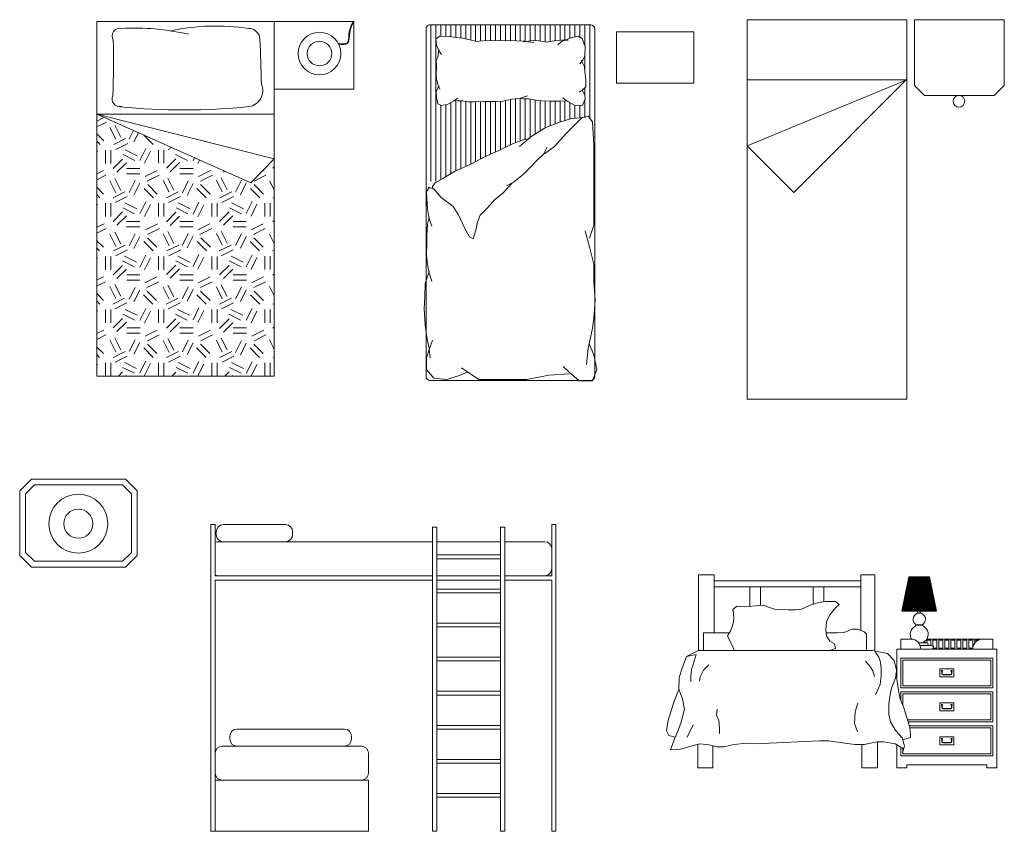
# Model space of a CAD drawing. Units: inches. Extents: x 1994 to 3075, y 3517 to 3950.
# Tile 4 of 58: x 1993.8976 to 1994.1162, y 3553.2299 to 3553.4101. Entities that reach past the tile are written whole.
import ezdxf

# ---------------------------------------------------------------- set-up
doc = ezdxf.new("R2010")
doc.units = ezdxf.units.IN
doc.layers.add('A-FURN-REFR', color=8, linetype='Continuous', lineweight=13)
doc.layers.add('A-FURN-REFR-PATT', color=8, linetype='Continuous', lineweight=13)

# ---------------------------------------------------------------- blocks, each defined once
blk = doc.blocks.new('*X4')
at = {"color": 0, "linetype": 'ByBlock'}
for p, q in [((19.525, 32.20386098788682), (19.525, 32.675)), ((19.55, 32.56810532391988), (19.55, 32.675)), ((19.575, 32.61302412421321), (19.575, 32.675)), ((19.6, 32.61427234615303), (19.6, 32.675)), ((19.625, 32.60794036333506), (19.625, 32.675)), ((19.65, 32.59793129896265), (19.65, 32.675)), ((19.675, 32.59817646525313), (19.675, 32.675)), ((19.7, 32.59593125927973), (19.7, 32.675)), ((19.725, 32.59071820491911), (19.725, 32.675)), ((19.75, 32.58875626807508), (19.75, 32.675)), ((19.775, 32.5935224892048), (19.775, 32.675)), ((19.8, 32.59614861867567), (19.8, 32.675)), ((19.825, 32.59455734515703), (19.825, 32.675)), ((19.85, 32.5927879885456), (19.85, 32.675)), ((19.875, 32.59404453025058), (19.875, 32.675)), ((19.9, 32.59519703632207), (19.9, 32.675)), ((19.925, 32.59638859160449), (19.925, 32.675)), ((19.95, 32.59617959359129), (19.95, 32.675)), ((19.975, 32.59528592712948), (19.975, 32.675)), ((20, 32.59564247452483), (20, 32.675)), ((20.025, 32.59653254351594), (20.025, 32.675)), ((20.05, 32.59544460173633), (20.05, 32.675)), ((20.075, 32.59363490203366), (20.075, 32.675)), ((20.1, 32.59241134187158), (20.1, 32.675)), ((20.125, 32.598098310265), (20.125, 32.675)), ((20.15, 32.60389733444189), (20.15, 32.675)), ((20.175, 32.60912913191685), (20.175, 32.675)), ((20.2, 32.61238895624688), (20.2, 32.675)), ((20.225, 32.61502292055541), (20.225, 32.675)), ((20.25, 32.61658776692677), (20.25, 32.675)), ((20.275, 32.61758867336402), (20.275, 32.675)), ((20.3, 32.60301153474566), (20.3, 32.675)), ((20.325, 32.44626119300636), (20.325, 32.675)), ((20.3, 32.44626119300636), (20.3, 32.59766660268327)), ((19.55, 32.43429497183709), (19.55, 32.5303145499151)), ((20.3, 31.8855920007165), (20.3, 32.44626119300636)), ((20.325, 31.8855920007165), (20.325, 32.44626119300636)), ((19.55, 32.31736883828921), (19.55, 32.3583983061656)), ((19.55, 32.21177313200482), (19.55, 32.29839776882886)), ((19.65, 32.19310101720963), (19.65, 32.29148655342231)), ((19.75, 32.1550408149583), (19.75, 32.29147480162358)), ((19.775, 32.14004617199367), (19.775, 32.2932065184746)), ((19.8, 32.12505152902905), (19.8, 32.29695991761424)), ((19.825, 32.10859105723152), (19.825, 32.30058402418693)), ((19.85, 32.09722511488017), (19.85, 32.30182870692274)), ((19.875, 32.08964787427039), (19.875, 32.30376454748067)), ((19.9, 32.08012334199107), (19.9, 32.30225038066949)), ((19.925, 32.06962839826795), (19.925, 32.2984329992773)), ((19.95, 32.05796084622579), (19.95, 32.29321994491666)), ((20.175, 31.95038486477602), (20.175, 32.2922523717346)), ((20.2, 31.93854186082345), (20.2, 32.29303571994302)), ((19.575, 32.20638032842688), (19.575, 32.26988957351553)), ((19.6, 32.20358354634456), (19.6, 32.27108112879796)), ((19.625, 32.20024132338327), (19.625, 32.28364984065946)), ((19.675, 32.18574866757895), (19.675, 32.29033710469695)), ((19.7, 32.17575223893587), (19.7, 32.29033710469695)), ((19.725, 32.16575581029279), (19.725, 32.29043219075145)), ((19.975, 32.04629329418363), (19.975, 32.28980448432189)), ((20, 32.03487552737632), (20, 32.28861292903947)), ((20.025, 32.02358434798068), (20.025, 32.28842183765934)), ((20.05, 32.01229316858503), (20.05, 32.28842183765934)), ((20.075, 31.99969466619798), (20.075, 32.28784730729937)), ((20.1, 31.98673071948447), (20.1, 32.2869205420797)), ((20.125, 31.97407087268117), (20.125, 32.28650657062169)), ((20.15, 31.9622278687286), (20.15, 32.28908964647222)), ((20.225, 31.92436703603548), (20.225, 32.28364705813529)), ((20.25, 31.90936589769556), (20.25, 32.27313805462554)), ((20.275, 31.89509549871252), (20.275, 32.27050875367903))]:
    blk.add_line(p, q, dxfattribs=at)

msp = doc.modelspace()

# ---------------------------------------------------------------- hatches: boundary and pattern name
at = {"layer": 'A-FURN-REFR-PATT'}
h = msp.add_hatch(dxfattribs=at)
h.set_pattern_fill('GEOL2', color=256, scale=0.0118110236220473, style=0, pattern_type=2)
h.set_pattern_definition([(0, (2000.169371235036, 3548.887718539946), (0.0118110236220473, 0.0118110236220473), [0.0029527559055118, -0.0088582677165354]), (0, (2000.169371235036, 3548.888899642308), (0.0118110236220473, 0.0118110236220473), [0.0029527559055118, -0.0088582677165354]), (90, (2000.176457849209, 3548.890080744671), (-0.0118110236220473, 0.0118110236220473), [0.0029527559055118, -0.0088582677165354]), (90, (2000.177638951571, 3548.890080744671), (-0.0118110236220473, 0.0118110236220473), [0.0029527559055118, -0.0088582677165354]), (45, (2000.178229502752, 3548.888899642308), (0, 0.011811023622272), [0.0029527559055118, -0.0137505538818898]), (45, (2000.179056274406, 3548.888072870655), (0, 0.011811023622272), [0.0029527559055118, -0.0137505538818898]), (135, (2000.175276746847, 3548.894214602938), (-0.011811023622272, 0), [0.0029527559055118, -0.0137505538818898]), (135, (2000.1761035185, 3548.895041374592), (-0.011811023622272, 0), [0.0029527559055118, -0.0137505538818898]), (26.56505119999999, (2000.178229502752, 3548.894214602938), (0.0118110236220484, 4.7252e-12), [0.0029527559055118, -0.0234574957913386]), (26.56505119999999, (2000.178701943697, 3548.893151610812), (0.0118110236220484, 4.7252e-12), [0.0029527559055118, -0.0234574957913386]), (26.56505119999999, (2000.173505093304, 3548.898939012387), (0.0118110236220484, 4.7252e-12), [0.0029527559055118, -0.0234574957913386]), (26.56505119999999, (2000.173977534248, 3548.897876020261), (0.0118110236220484, 4.7252e-12), [0.0029527559055118, -0.0234574957913386]), (63.43494882000001, (2000.172323990941, 3548.890671295851), (6.023e-13, 0.0118110236220484), [0.0029527559055118, -0.0234574957913385]), (63.43494882000001, (2000.173386983067, 3548.890080744671), (6.023e-13, 0.0118110236220484), [0.0029527559055118, -0.0234574957913385]), (63.43494882000001, (2000.171024778343, 3548.894805154119), (6.023e-13, 0.0118110236220484), [0.0029527559055118, -0.0234574957913385]), (63.43494882000001, (2000.169961786217, 3548.8953957053), (6.023e-13, 0.0118110236220484), [0.0029527559055118, -0.0234574957913385]), (116.5650512, (2000.179883046059, 3548.895868146245), (-4.7252e-12, 0.0118110236220484), [0.0029527559055118, -0.0234574957913386]), (116.5650512, (2000.178820053934, 3548.8953957053), (-4.7252e-12, 0.0118110236220484), [0.0029527559055118, -0.0234574957913386]), (153.43494882, (2000.171142888579, 3548.890671295851), (-0.0118110236220484, 6.024e-13), [0.0029527559055118, -0.0234574957913386]), (153.43494882, (2000.171615329524, 3548.891734287977), (-0.0118110236220484, 6.024e-13), [0.0029527559055118, -0.0234574957913386])])
h.paths.add_polyline_path([(1993.954109154694, 3553.379219006938), (1993.948922264658, 3553.373891692003), (1993.914739075954, 3553.389155305615), (1993.914739075954, 3553.330989736288), (1993.954109154694, 3553.330989736288)])
h = msp.add_hatch(dxfattribs=at)
h.set_pattern_fill('ANSI38', color=256, scale=7.66347049375e-05, angle=90, style=0)
h.set_pattern_definition([(135, (0, 0), (-0.0001720498195254, -0.0001720498195254), []), (225, (0, 0), (-0.0001720498195254, -0.0005161494585763), [0.0006082879704418, -0.0003649727822651])])
h.paths.add_polyline_path([(1994.099628953712, 3553.286448017916), (1994.10116164781, 3553.278784547428), (1994.093498177321, 3553.278784547428), (1994.095030871418, 3553.286448017916)])

# ---------------------------------------------------------------- linework, layer by layer
at = {"layer": 'A-FURN-REFR'}
for p, q in [((1993.954109154694, 3553.409729893769), (1993.914739075954, 3553.409729893769)), ((1993.914739075954, 3553.409729893769), (1993.914739075954, 3553.330989736288)), ((1993.954109154694, 3553.394673371351), (1993.954109154694, 3553.409729893769)), ((1993.954109154694, 3553.409729893769), (1993.971825690127, 3553.409729893769)), ((1993.971825690127, 3553.409729893769), (1993.971825690127, 3553.394673371351)), ((1994.059155926548, 3553.325914112681), (1994.059155926548, 3553.410067655988)), ((1994.059155926548, 3553.410067655988), (1994.094588997414, 3553.410067655988)), ((1994.094588997414, 3553.410067655988), (1994.094588997414, 3553.325914112681)), ((1994.0962845141, 3553.410135377998), (1994.116215616461, 3553.410135377998)), ((1994.0962845141, 3553.410135377998), (1994.0962845141, 3553.395519236266)), ((1994.116215616461, 3553.410135377998), (1994.116215616461, 3553.395519236266)), ((1994.059155926548, 3553.396780254413), (1994.094588997414, 3553.396780254413)), ((1994.094588997414, 3553.396780254413), (1994.059155926548, 3553.382103395904)), ((1994.09458426814, 3553.396915934153), (1994.06946382822, 3553.371795494232)), ((1994.094588997414, 3553.396780254413), (1994.094588997414, 3553.396780254413)), ((1994.094588997414, 3553.396780254413), (1994.094588997414, 3553.396780254413)), ((1994.094588997414, 3553.396780254413), (1994.094588997414, 3553.396780254413)), ((1993.971825690127, 3553.394673371351), (1993.954109154694, 3553.394673371351)), ((1993.954109154694, 3553.330989736288), (1993.954109154694, 3553.394673371351)), ((1994.098499081028, 3553.393304669337), (1994.0962845141, 3553.395519236266)), ((1994.114001049533, 3553.393304669337), (1994.116215616461, 3553.395519236266)), ((1994.098499081028, 3553.393304669337), (1994.114001049533, 3553.393304669337)), ((1993.914739075954, 3553.389155305615), (1993.948922264658, 3553.373891692003)), ((1993.914739075954, 3553.389155305615), (1993.954119737166, 3553.379216336113)), ((1993.954109154694, 3553.389155305615), (1993.914739075954, 3553.389155305615)), ((1994.059155926548, 3553.382103395904), (1994.06946382822, 3553.371795494232)), ((1993.948922264658, 3553.373891692003), (1993.954109154694, 3553.379219006938)), ((1993.914739075954, 3553.330989736288), (1993.954109154694, 3553.330989736288)), ((1994.094588997414, 3553.325914112681), (1994.059155926548, 3553.325914112681)), ((1993.900243127395, 3553.308154526741), (1993.897632269542, 3553.305543668888)), ((1993.900895841858, 3553.306849097815), (1993.898937698468, 3553.304890954425)), ((1993.921129990221, 3553.308154526741), (1993.900243127395, 3553.308154526741)), ((1993.920477275758, 3553.306849097815), (1993.900895841858, 3553.306849097815)), ((1993.922435419148, 3553.304890954425), (1993.920477275758, 3553.306849097815)), ((1993.923740848074, 3553.305543668888), (1993.921129990221, 3553.308154526741)), ((1993.897632269542, 3553.305543668888), (1993.897632269542, 3553.291183950694)), ((1993.898937698468, 3553.304890954425), (1993.898937698468, 3553.291836665158)), ((1993.922435419148, 3553.291836665158), (1993.922435419148, 3553.304890954425)), ((1993.923740848074, 3553.291183950694), (1993.923740848074, 3553.305543668888)), ((1993.989260282976, 3553.297440995406), (1993.990205889731, 3553.297440995406)), ((1994.004404726865, 3553.297440995406), (1994.005350333621, 3553.297440995406)), ((1993.897632269542, 3553.291183950694), (1993.900243127395, 3553.288573092841)), ((1993.898937698468, 3553.291836665158), (1993.900895841858, 3553.289878521769)), ((1993.920477275758, 3553.289878521769), (1993.922435419148, 3553.291836665158)), ((1993.921129990221, 3553.288573092841), (1993.923740848074, 3553.291183950694)), ((1993.900895841858, 3553.289878521769), (1993.920477275758, 3553.289878521769)), ((1993.900243127395, 3553.288573092841), (1993.921129990221, 3553.288573092841)), ((1994.051841460532, 3553.286859217838), (1994.048294257176, 3553.286859217838)), ((1994.048294257176, 3553.286859217838), (1994.048294257176, 3553.27005170713)), ((1994.051841460532, 3553.274014635587), (1994.051841460532, 3553.286859217838)), ((1994.084390635564, 3553.274536402606), (1994.084390635564, 3553.286859217838)), ((1994.084390635564, 3553.286859217838), (1994.087457124975, 3553.286859217838)), ((1994.087457124975, 3553.286859217838), (1994.087457124975, 3553.269935694535)), ((1994.051841460532, 3553.285558051226), (1994.084390635564, 3553.285558051226)), ((1994.093498177321, 3553.278784547427), (1994.095030871418, 3553.286448017916)), ((1994.099628953712, 3553.286448017916), (1994.095030871418, 3553.286448017916)), ((1994.099628953712, 3553.286448017916), (1994.10116164781, 3553.278784547427)), ((1994.084390635564, 3553.284195219957), (1994.051841460532, 3553.284195219957)), ((1994.059755020064, 3553.284195219957), (1994.059755020064, 3553.279932083761)), ((1994.062088181079, 3553.284195219957), (1994.062088181079, 3553.280069509611)), ((1994.073807242988, 3553.284195219957), (1994.073807242988, 3553.280381305924)), ((1994.076140404003, 3553.284195219957), (1994.076140404003, 3553.280903425881)), ((1994.058479080529, 3553.279808747126), (1994.062797378561, 3553.280120750106)), ((1994.062797378561, 3553.280120750106), (1994.063629812153, 3553.279808747126)), ((1994.072006255235, 3553.279652745637), (1994.073098841809, 3553.28017275422)), ((1994.073098841809, 3553.28017275422), (1994.075053706907, 3553.280748262081)), ((1994.075053706907, 3553.280748262081), (1994.076510484098, 3553.280956267685)), ((1994.076510484098, 3553.280956267685), (1994.07874766134, 3553.280956267685)), ((1994.07874766134, 3553.280956267685), (1994.079580109657, 3553.280280257612)), ((1994.079580109657, 3553.280280257612), (1994.07874766134, 3553.279552232571)), ((1994.055981765029, 3553.279184730314), (1994.056866232162, 3553.279912744502)), ((1994.056085817387, 3553.278352707899), (1994.055981765029, 3553.279184730314)), ((1994.056137850929, 3553.277000676899), (1994.056085817387, 3553.278352707899)), ((1994.056866232162, 3553.279912744502), (1994.058479080529, 3553.279808747126)), ((1994.063629812153, 3553.279808747126), (1994.065190641703, 3553.279288727689)), ((1994.065190641703, 3553.279288727689), (1994.066751471252, 3553.279184730314)), ((1994.066751471252, 3553.279184730314), (1994.068260267261, 3553.279080722085)), ((1994.068260267261, 3553.279080722085), (1994.069873130351, 3553.279080722085)), ((1994.069873130351, 3553.279080722085), (1994.07122584046, 3553.279288727689)), ((1994.07122584046, 3553.279288727689), (1994.072006255235, 3553.279652745637)), ((1994.077446970049, 3553.277992195968), (1994.076718588815, 3553.276432159364)), ((1994.07874766134, 3553.279552232571), (1994.077446970049, 3553.277992195968)), ((1994.10116164781, 3553.278784547427), (1994.093498177321, 3553.278784547427)), ((1994.055409454971, 3553.274400612276), (1994.055929731487, 3553.275752643275)), ((1994.055929731487, 3553.275752643275), (1994.056137850929, 3553.277000676899)), ((1994.076718588815, 3553.276432159364), (1994.076562502916, 3553.274664117156)), ((1994.098128450965, 3553.275752817065), (1994.096531374166, 3553.275752817065)), ((1994.098128450965, 3553.275671139821), (1994.096531374166, 3553.275671139821)), ((1994.09812626846, 3553.275711978443), (1994.096533556671, 3553.275711978443)), ((1994.049432288437, 3553.27005170713), (1994.049432288437, 3553.274014635587)), ((1994.049432288437, 3553.274014635587), (1994.055170395957, 3553.274014635587)), ((1994.054733092555, 3553.27330858014), (1994.055409454971, 3553.274400612276)), ((1994.076562502916, 3553.274664117156), (1994.076770622356, 3553.273364079418)), ((1994.076666562636, 3553.274014098287), (1994.079147556919, 3553.273976101961)), ((1994.079147556919, 3553.273976101961), (1994.080664421513, 3553.274107941238)), ((1994.080664421513, 3553.274107941238), (1994.082445090566, 3553.274833035553)), ((1994.082445090566, 3553.274833035553), (1994.083698150701, 3553.274833035553)), ((1994.083698150701, 3553.274833035553), (1994.085083120427, 3553.27423976966)), ((1994.085083120427, 3553.27423976966), (1994.085610729344, 3553.27371243426)), ((1994.085610729344, 3553.27371243426), (1994.085610729344, 3553.272262245631)), ((1994.056293922104, 3553.27005170713), (1994.054733092555, 3553.27330858014)), ((1994.076770622356, 3553.273364079418), (1994.07749900359, 3553.272168049908)), ((1994.07749900359, 3553.272168049908), (1994.078487523082, 3553.271544033096)), ((1994.078487523082, 3553.271544033096), (1994.07874766134, 3553.270504005076)), ((1994.085610729344, 3553.272262245631), (1994.085610729344, 3553.27005170713)), ((1994.093238606363, 3553.272626038975), (1994.095456045741, 3553.272626038975)), ((1994.093238606363, 3553.272626038975), (1994.093238606363, 3553.270408599597)), ((1994.097192198074, 3553.271788024285), (1994.099015876073, 3553.271788024285)), ((1994.09856046087, 3553.27208270374), (1994.09856046087, 3553.271788024285)), ((1994.099003948745, 3553.271788024285), (1994.099003948745, 3553.272404295037)), ((1994.099003948745, 3553.272404295037), (1994.099890924496, 3553.272404295037)), ((1994.111421609261, 3553.272626038975), (1994.099039287332, 3553.272626038975)), ((1994.099890924496, 3553.272404295037), (1994.099890924496, 3553.271174946646)), ((1994.100334412372, 3553.271085844229), (1994.100334412372, 3553.272404295037)), ((1994.100334412372, 3553.272404295037), (1994.101221388123, 3553.272404295037)), ((1994.101221388123, 3553.272404295037), (1994.101221388123, 3553.270630343535)), ((1994.101664875999, 3553.270630343535), (1994.101664875999, 3553.272404295037)), ((1994.101664875999, 3553.272404295037), (1994.10255185175, 3553.272404295037)), ((1994.10255185175, 3553.272404295037), (1994.10255185175, 3553.270630343535)), ((1994.102995339625, 3553.270630343535), (1994.102995339625, 3553.272404295037)), ((1994.102995339625, 3553.272404295037), (1994.103882315376, 3553.272404295037)), ((1994.103882315376, 3553.272404295037), (1994.103882315376, 3553.270630343535)), ((1994.105212779003, 3553.272404295037), (1994.104325803252, 3553.272404295037)), ((1994.104325803252, 3553.272404295037), (1994.104325803252, 3553.270630343535)), ((1994.105212779003, 3553.270630343535), (1994.105212779003, 3553.272404295037)), ((1994.10654324263, 3553.272404295037), (1994.105656266879, 3553.272404295037)), ((1994.105656266879, 3553.272404295037), (1994.105656266879, 3553.270630343535)), ((1994.10654324263, 3553.270630343535), (1994.10654324263, 3553.272404295037)), ((1994.107873706257, 3553.272404295037), (1994.106986730505, 3553.272404295037)), ((1994.106986730505, 3553.272404295037), (1994.106986730505, 3553.270630343535)), ((1994.107873706257, 3553.270630343535), (1994.107873706257, 3553.272404295037)), ((1994.109204169883, 3553.272404295037), (1994.108317194132, 3553.272404295037)), ((1994.108317194132, 3553.272404295037), (1994.108317194132, 3553.270630343535)), ((1994.109204169883, 3553.270630343535), (1994.109204169883, 3553.272404295037)), ((1994.110455049845, 3553.272404295037), (1994.109647657759, 3553.272404295037)), ((1994.109647657759, 3553.272404295037), (1994.109647657759, 3553.271739063224)), ((1994.111421609261, 3553.272626038975), (1994.113639048639, 3553.272626038975)), ((1994.113639048639, 3553.272626038975), (1994.113639048639, 3553.270408599597)), ((1994.045634156494, 3553.268737970959), (1994.048294257176, 3553.27005170713)), ((1994.045634156494, 3553.268737970959), (1994.047835731839, 3553.269193232193)), ((1994.047835731839, 3553.269193232193), (1994.047152478733, 3553.266992777564)), ((1994.048294257176, 3553.27005170713), (1994.086917560417, 3553.27005170713)), ((1994.07874766134, 3553.270504005076), (1994.077417699342, 3553.27005170713)), ((1994.086917560417, 3553.27005170713), (1994.087980390402, 3553.269823186441)), ((1994.087448975409, 3553.269937446786), (1994.088359967281, 3553.26860913839)), ((1994.087980390402, 3553.269823186441), (1994.090308641991, 3553.269405505543)), ((1994.090308641991, 3553.269405505543), (1994.091776203363, 3553.267850351574)), ((1994.092351630612, 3553.270408599597), (1994.092351630612, 3553.263805254229)), ((1994.092351630612, 3553.270408599597), (1994.11452602439, 3553.270408599597)), ((1994.097536850776, 3553.271174946646), (1994.100088761942, 3553.271174946646)), ((1994.097673485119, 3553.270408599597), (1994.097673485119, 3553.270408599597)), ((1994.101221388123, 3553.270630343535), (1994.100436270846, 3553.270630343535)), ((1994.10255185175, 3553.270630343535), (1994.101664875999, 3553.270630343535)), ((1994.103882315376, 3553.270630343535), (1994.102995339625, 3553.270630343535)), ((1994.104325803252, 3553.270630343535), (1994.105212779003, 3553.270630343535)), ((1994.105656266879, 3553.270630343535), (1994.10654324263, 3553.270630343535)), ((1994.106986730505, 3553.270630343535), (1994.107873706257, 3553.270630343535)), ((1994.108317194132, 3553.270630343535), (1994.109204169883, 3553.270630343535)), ((1994.109204169883, 3553.270408599597), (1994.109204169883, 3553.270408599597)), ((1994.11452602439, 3553.270408599597), (1994.11452602439, 3553.244026942197)), ((1994.044647256609, 3553.265930486877), (1994.045634156494, 3553.268737970959)), ((1994.047152478733, 3553.266992777564), (1994.046772901855, 3553.265854602768)), ((1994.050594363494, 3553.26688483999), (1994.049399844773, 3553.265690927116)), ((1994.086386152786, 3553.266636314378), (1994.085399238177, 3553.267698605065)), ((1994.088359967281, 3553.26860913839), (1994.08873954416, 3553.267470963593)), ((1994.08873954416, 3553.267470963593), (1994.088891389635, 3553.266029284924)), ((1994.091776203363, 3553.267850351574), (1994.092307610993, 3553.265725781053)), ((1994.093238606363, 3553.268412904157), (1994.113639048639, 3553.268412904157)), ((1994.093238606363, 3553.261760586023), (1994.093238606363, 3553.268412904157)), ((1994.093682094239, 3553.262204073899), (1994.093682094239, 3553.267969416282)), ((1994.093682094239, 3553.267969416282), (1994.113195560763, 3553.267969416282)), ((1994.113195560763, 3553.267969416282), (1994.113195560763, 3553.262204073899)), ((1994.113639048639, 3553.268412904157), (1994.113639048639, 3553.261760586023)), ((1994.044039918878, 3553.264109420227), (1994.044647256609, 3553.265930486877)), ((1994.046772901855, 3553.265854602768), (1994.046621071103, 3553.264261166736)), ((1994.049399844773, 3553.265690927116), (1994.048708272779, 3553.264245666448)), ((1994.086993475793, 3553.26557402369), (1994.086386152786, 3553.266636314378)), ((1994.087373052671, 3553.26428409153), (1994.086993475793, 3553.26557402369)), ((1994.088891389635, 3553.266029284924), (1994.088891389635, 3553.264359975639)), ((1994.092307610993, 3553.265725781053), (1994.092079864866, 3553.26390470355)), ((1994.09219373793, 3553.264815242302), (1994.092763117972, 3553.261173103576)), ((1994.101886619936, 3553.265973720841), (1994.104991035065, 3553.265973720841)), ((1994.101886619936, 3553.264199769339), (1994.101886619936, 3553.265973720841)), ((1994.102330107812, 3553.264953698727), (1994.102330107812, 3553.265530232965)), ((1994.102330107812, 3553.265530232965), (1994.102418805387, 3553.265530232965)), ((1994.102418805387, 3553.264953698727), (1994.102418805387, 3553.265530232965)), ((1994.104237105677, 3553.26473195479), (1994.102640549325, 3553.26473195479)), ((1994.104458849615, 3553.265530232965), (1994.10454754719, 3553.265530232965)), ((1994.104458849615, 3553.265530232965), (1994.104458849615, 3553.264953698727)), ((1994.10454754719, 3553.265530232965), (1994.10454754719, 3553.264953698727)), ((1994.104991035065, 3553.265973720841), (1994.104991035065, 3553.264199769339)), ((1994.043964003503, 3553.261529566762), (1994.044039918878, 3553.264109420227)), ((1994.046621071103, 3553.264261166736), (1994.046621071103, 3553.263198876049)), ((1994.048708272779, 3553.264245666448), (1994.04858254714, 3553.263303101368)), ((1994.088663628784, 3553.26253890899), (1994.087600813523, 3553.260262570251)), ((1994.088891389635, 3553.264359975639), (1994.088663628784, 3553.26253890899)), ((1994.092079864866, 3553.26390470355), (1994.091168865633, 3553.26170424892)), ((1994.104991035065, 3553.264199769339), (1994.101886619936, 3553.264199769339)), ((1994.104237105677, 3553.264643257215), (1994.102640549325, 3553.264643257215)), ((1994.043964003503, 3553.261529566762), (1994.042861434263, 3553.258590286822)), ((1994.04479908736, 3553.259329112132), (1994.043964003503, 3553.261529566762)), ((1994.091168865633, 3553.26170424892), (1994.090789288754, 3553.259883182271)), ((1994.092763117972, 3553.261173103576), (1994.093066779475, 3553.259352036927)), ((1994.093238606363, 3553.261760586023), (1994.113639048639, 3553.261760586023)), ((1994.093238606363, 3553.258946101423), (1994.093238606363, 3553.260873610272)), ((1994.093238606363, 3553.260873610272), (1994.113639048639, 3553.260873610272)), ((1994.093682094239, 3553.262204073899), (1994.113195560763, 3553.262204073899)), ((1994.093682094239, 3553.260430122396), (1994.113195560763, 3553.260430122396)), ((1994.093682094239, 3553.257898375558), (1994.093682094239, 3553.260430122396)), ((1994.113195560763, 3553.260430122396), (1994.113195560763, 3553.254664780014)), ((1994.113639048639, 3553.260873610272), (1994.113639048639, 3553.254221292139)), ((1994.042861434263, 3553.258590286822), (1994.041604060084, 3553.254505852612)), ((1994.045254579615, 3553.257052773394), (1994.04479908736, 3553.259329112132)), ((1994.083729070462, 3553.258365619494), (1994.083121747456, 3553.256468668736)), ((1994.090789288754, 3553.259883182271), (1994.090561542627, 3553.258137988876)), ((1994.090561542627, 3553.258137988876), (1994.090561542627, 3553.255861650138)), ((1994.093066779475, 3553.259352036927), (1994.093901848609, 3553.257379212915)), ((1994.101886619936, 3553.256660475454), (1994.101886619936, 3553.258434426957)), ((1994.101886619936, 3553.258434426957), (1994.104991035065, 3553.258434426957)), ((1994.104991035065, 3553.258434426957), (1994.104991035065, 3553.256660475454)), ((1994.044419495758, 3553.253941774585), (1994.045254579615, 3553.257052773394)), ((1994.052354699122, 3553.255699765486), (1994.052480439485, 3553.257082189205)), ((1994.083121747456, 3553.256468668736), (1994.082969916705, 3553.253888826125)), ((1994.093901848609, 3553.257379212915), (1994.095192424721, 3553.253281807527)), ((1994.104991035065, 3553.256660475454), (1994.101886619936, 3553.256660475454)), ((1994.102330107812, 3553.25799093908), (1994.102418805387, 3553.25799093908)), ((1994.102330107812, 3553.257414404843), (1994.102330107812, 3553.25799093908)), ((1994.102418805387, 3553.257414404843), (1994.102418805387, 3553.25799093908)), ((1994.104237105677, 3553.257192660905), (1994.102640549325, 3553.257192660905)), ((1994.104237105677, 3553.25710396333), (1994.102640549325, 3553.25710396333)), ((1994.104458849615, 3553.25799093908), (1994.104458849615, 3553.257414404843)), ((1994.104458849615, 3553.25799093908), (1994.10454754719, 3553.25799093908)), ((1994.10454754719, 3553.25799093908), (1994.10454754719, 3553.257414404843)), ((1994.041604060084, 3553.254505852612), (1994.041226838997, 3553.252243700761)), ((1994.043508511248, 3553.251665446701), (1994.044419495758, 3553.253941774585)), ((1994.052857645849, 3553.254505852612), (1994.052354699122, 3553.255699765486)), ((1994.052983386211, 3553.252809244151), (1994.052857645849, 3553.254505852612)), ((1994.082969916705, 3553.253888826125), (1994.083653155087, 3553.251991875367)), ((1994.090561542627, 3553.255861650138), (1994.090941119505, 3553.254268214106)), ((1994.090941119505, 3553.254268214106), (1994.092155780242, 3553.25221951684)), ((1994.094756824363, 3553.254664780014), (1994.113195560763, 3553.254664780014)), ((1994.094896511507, 3553.254221292139), (1994.113639048639, 3553.254221292139)), ((1994.041226838997, 3553.252243700761), (1994.041729800447, 3553.251238309587)), ((1994.042825258142, 3553.249996126561), (1994.043508511248, 3553.251665446701)), ((1994.047136547695, 3553.253563287532), (1994.045816288611, 3553.250861277041)), ((1994.052983386211, 3553.251678168225), (1994.052983386211, 3553.252809244151)), ((1994.092155780242, 3553.25221951684), (1994.092155780242, 3553.25221951684)), ((1994.092155780242, 3553.25221951684), (1994.09352227173, 3553.250701954063)), ((1994.095175885796, 3553.253334316388), (1994.113639048639, 3553.253334316388)), ((1994.095192424721, 3553.253281807527), (1994.095420185572, 3553.251688371496)), ((1994.09524831006, 3553.252890828512), (1994.113195560763, 3553.252890828512)), ((1994.095420185572, 3553.251688371496), (1994.095420185572, 3553.250777827317)), ((1994.113195560763, 3553.252890828512), (1994.113195560763, 3553.247125486129)), ((1994.113639048639, 3553.253334316388), (1994.113639048639, 3553.246681998254)), ((1994.041729800447, 3553.251238309587), (1994.041729800447, 3553.251238309587)), ((1994.041729800447, 3553.251238309587), (1994.043166884695, 3553.250830786631)), ((1994.042142019759, 3553.248023302549), (1994.042825258142, 3553.249996126561)), ((1994.045816288611, 3553.250861277041), (1994.045816288611, 3553.250861277041)), ((1994.048594900321, 3553.249389107963), (1994.047759816464, 3553.249161466491)), ((1994.050644630192, 3553.249161466491), (1994.048594900321, 3553.249389107963)), ((1994.059071339971, 3553.249540865326), (1994.056186526243, 3553.2492373506)), ((1994.0608265812, 3553.249389107963), (1994.059071339971, 3553.249540865326)), ((1994.059071339971, 3553.249540865326), (1994.059071339971, 3553.249540865326)), ((1994.075153945829, 3553.250019051355), (1994.0608265812, 3553.249389107963)), ((1994.077276189901, 3553.250019051355), (1994.075153945829, 3553.250019051355)), ((1994.080312849104, 3553.24956379012), (1994.077276189901, 3553.250019051355)), ((1994.08304583208, 3553.249184391285), (1994.080312849104, 3553.24956379012)), ((1994.086841645041, 3553.24956379012), (1994.08517149205, 3553.249184391285)), ((1994.088056305778, 3553.249791420738), (1994.086841645041, 3553.24956379012)), ((1994.089422797266, 3553.249791420738), (1994.088056305778, 3553.249791420738)), ((1994.088056305778, 3553.249791420738), (1994.088056305778, 3553.244026942197)), ((1994.09200394949, 3553.249336148648), (1994.089422797266, 3553.249791420738)), ((1994.09352227173, 3553.250701954063), (1994.094053694084, 3553.248805003305)), ((1994.095420185572, 3553.250777827317), (1994.093640674913, 3553.250279305286)), ((1994.101886619936, 3553.250895133072), (1994.104991035065, 3553.250895133072)), ((1994.101886619936, 3553.24912118157), (1994.101886619936, 3553.250895133072)), ((1994.102330107812, 3553.249875110958), (1994.102330107812, 3553.250451645197)), ((1994.102330107812, 3553.250451645197), (1994.102418805387, 3553.250451645197)), ((1994.102418805387, 3553.249875110958), (1994.102418805387, 3553.250451645197)), ((1994.104237105677, 3553.249653367021), (1994.102640549325, 3553.249653367021)), ((1994.104237105677, 3553.249564669445), (1994.102640549325, 3553.249564669445)), ((1994.104458849615, 3553.250451645197), (1994.10454754719, 3553.250451645197)), ((1994.104458849615, 3553.250451645197), (1994.104458849615, 3553.249875110958)), ((1994.10454754719, 3553.250451645197), (1994.10454754719, 3553.249875110958)), ((1994.104991035065, 3553.250895133072), (1994.104991035065, 3553.24912118157)), ((1994.044343580382, 3553.248175059912), (1994.042142019759, 3553.248023302549)), ((1994.047759816464, 3553.249161466491), (1994.044343580382, 3553.248175059912)), ((1994.048142396977, 3553.244026942197), (1994.048142396977, 3553.249265756845)), ((1994.052390713282, 3553.248706205256), (1994.050644630192, 3553.249161466491)), ((1994.051517671737, 3553.248933835873), (1994.051517671737, 3553.244026942197)), ((1994.053984950897, 3553.248706205256), (1994.052390713282, 3553.248706205256)), ((1994.056186526243, 3553.2492373506), (1994.053984950897, 3553.248706205256)), ((1994.08517149205, 3553.249184391285), (1994.08304583208, 3553.249184391285)), ((1994.084594558752, 3553.244026942197), (1994.084594558752, 3553.249184391285)), ((1994.093863898283, 3553.248235921333), (1994.09200394949, 3553.249336148648)), ((1994.092351630612, 3553.249130482628), (1994.092351630612, 3553.244026942197)), ((1994.093238606363, 3553.246681998254), (1994.093238606363, 3553.248605804232)), ((1994.094053694084, 3553.248805003305), (1994.093674102481, 3553.247666839363)), ((1994.093674102481, 3553.247666839363), (1994.093863898283, 3553.248235921333)), ((1994.093674102481, 3553.247666839363), (1994.093674102481, 3553.247666839363)), ((1994.093682094239, 3553.247125486129), (1994.093682094239, 3553.248343465034)), ((1994.104991035065, 3553.24912118157), (1994.101886619936, 3553.24912118157)), ((1994.093238606363, 3553.246681998254), (1994.113639048639, 3553.246681998254)), ((1994.093682094239, 3553.247125486129), (1994.113195560763, 3553.247125486129)), ((1994.051517671737, 3553.244026942197), (1994.048142396977, 3553.244026942197)), ((1994.088056305778, 3553.244026942197), (1994.084594558752, 3553.244026942197)), ((1994.094569069989, 3553.244026942197), (1994.092351630612, 3553.244026942197)), ((1994.094569069989, 3553.244686302814), (1994.094569069989, 3553.244026942197)), ((1994.094569069989, 3553.244686302814), (1994.112308585012, 3553.244686302814)), ((1994.112308585012, 3553.244686302814), (1994.112308585012, 3553.244026942197)), ((1994.112308585012, 3553.244026942197), (1994.11452602439, 3553.244026942197)), ((1993.990205889731, 3553.229935414131), (1993.989260282976, 3553.229935414131)), ((1994.005350333621, 3553.229935414131), (1994.004404726865, 3553.229935414131))]:
    msp.add_line(p, q, dxfattribs=at)
at = {"layer": 'A-FURN-REFR', "extrusion": (2.7404770908e-06, 0, 0.9999999999962449)}
for p, q in [((1994.017663083944, 3553.38745919332, -8.1741843e-08), (1994.014434587808, 3553.38616825607, -7.28942233e-08)), ((1994.019923031239, 3553.388104661945, -8.79351768e-08), (1994.017663083944, 3553.38745919332, -8.1741843e-08)), ((1994.023328786101, 3553.388485668112, -9.726857e-08), (1994.019923031239, 3553.388104661945, -8.79351768e-08)), ((1994.014434587808, 3553.38616825607, -7.28942233e-08), (1994.011206091673, 3553.384231850195, -6.40466036e-08)), ((1994.011206091673, 3553.384231850195, -6.40466036e-08), (1994.008623294764, 3553.381972710007, -5.69685079e-08))]:
    msp.add_line(p, q, dxfattribs=at)
at = {"layer": 'A-FURN-REFR', "extrusion": (0, 1, 2e-16)}
for p, q in [((1993.940088731704, 3553.298019100508), (1993.940088731704, 3553.229935414131)), ((1993.941034338459, 3553.298019100508), (1993.940088731704, 3553.298019100508)), ((1993.941034338459, 3553.298019100508), (1993.941034338459, 3553.286671819445)), ((1993.956634404617, 3553.298019100508), (1993.942837110295, 3553.298019100508)), ((1994.016682878878, 3553.298019100508), (1994.015737272123, 3553.298019100508)), ((1994.015737272123, 3553.298019100508), (1994.015737272123, 3553.286671819445)), ((1994.016682878878, 3553.229935414131), (1994.016682878878, 3553.298019100508)), ((1993.941252782606, 3553.29643477282), (1993.941252782606, 3553.295821001176)), ((1993.958218732305, 3553.295821001176), (1993.958218732305, 3553.29643477282)), ((1993.989260282976, 3553.297440995406), (1993.989260282976, 3553.285726212691)), ((1993.990205889731, 3553.229935414131), (1993.990205889731, 3553.297440995406)), ((1994.005350333621, 3553.297440995406), (1994.004404726865, 3553.297440995406)), ((1994.004404726865, 3553.297440995406), (1994.004404726865, 3553.285148107588)), ((1994.005350333621, 3553.229935414131), (1994.005350333621, 3553.297440995406)), ((1993.989260282976, 3553.294236673487), (1993.941673059392, 3553.294236673487)), ((1994.004404726865, 3553.294236673487), (1993.990205889731, 3553.294236673487)), ((1994.014152944435, 3553.294236673487), (1994.005350333621, 3553.294236673487)), ((1993.989260282976, 3553.286671819445), (1993.941034338459, 3553.286671819445)), ((1994.004404726865, 3553.286671819445), (1993.990205889731, 3553.286671819445)), ((1994.015737272123, 3553.286671819445), (1994.005350333621, 3553.286671819445)), ((1993.941034338459, 3553.247263221547), (1993.941034338459, 3553.285726212691)), ((1993.989260282976, 3553.285726212691), (1993.941034338459, 3553.285726212691)), ((1993.989260282976, 3553.229935414131), (1993.989260282976, 3553.285726212691)), ((1994.004404726865, 3553.285726212691), (1993.990205889731, 3553.285726212691)), ((1994.004404726865, 3553.229935414131), (1994.004404726865, 3553.285148107588)), ((1994.015737272123, 3553.285726212691), (1994.005350333621, 3553.285726212691)), ((1994.015737272123, 3553.229935414131), (1994.015737272123, 3553.285726212691)), ((1993.969714715081, 3553.252629976257), (1993.945856170473, 3553.252629976257)), ((1993.944271842785, 3553.251045648568), (1993.944271842785, 3553.250431876924)), ((1993.97129904277, 3553.250431876924), (1993.97129904277, 3553.251045648568)), ((1993.941034338459, 3553.247263221547), (1993.941034338459, 3553.242867022882)), ((1993.973491853959, 3553.248847549236), (1993.942618666147, 3553.248847549236)), ((1993.975076181648, 3553.242867022882), (1993.975076181648, 3553.247263221547)), ((1993.941034338459, 3553.241282695193), (1993.941034338459, 3553.242867022882)), ((1993.941034338459, 3553.229935414131), (1993.941034338459, 3553.241282695193)), ((1993.975076181648, 3553.241282695193), (1993.941034338459, 3553.241282695193)), ((1993.975076181648, 3553.229935414131), (1993.975076181648, 3553.241282695193)), ((1993.940088731704, 3553.229935414131), (1993.941034338459, 3553.229935414131)), ((1993.941034338459, 3553.229935414131), (1993.975076181648, 3553.229935414131)), ((1994.016682878878, 3553.229935414131), (1994.015737272123, 3553.229935414131))]:
    msp.add_line(p, q, dxfattribs=at)
at = {"layer": 'A-FURN-REFR', "extrusion": (2.7404770908e-06, 0, 0.9999999999962449), "elevation": 0.0054644779825559}
msp.add_lwpolyline([(1993.988716837792, 3553.330030000304, -0.4142135623730951), (1993.987835480637, 3553.330911357459), (1993.987835480637, 3553.408105389229, -0.4142135623730951), (1993.988716837792, 3553.408986746385), (1994.024411802563, 3553.408986746385, -0.4142135623730948), (1994.025293159718, 3553.408105389229), (1994.025293159718, 3553.330911357459, -0.4142135623730948), (1994.024411802563, 3553.330030000304)], format="xyb", close=True, dxfattribs=at)
at = {"layer": 'A-FURN-REFR'}
for points in [[(1994.030126135478, 3553.407469052605), (1994.047254692625, 3553.407469052605), (1994.047254692625, 3553.396026679955), (1994.030126135478, 3553.396026679955)], [(1993.990205889731, 3553.290454246467), (1994.004404726865, 3553.290454246467), (1994.004404726865, 3553.291285674671), (1993.990205889731, 3553.291285674671)], [(1993.990205889731, 3553.282889392425), (1994.004404726865, 3553.282889392425), (1994.004404726865, 3553.28372082063), (1993.990205889731, 3553.28372082063)], [(1993.990205889731, 3553.275324538383), (1994.004404726865, 3553.275324538383), (1994.004404726865, 3553.276155966587), (1993.990205889731, 3553.276155966587)], [(1993.990205889731, 3553.267759684341), (1994.004404726865, 3553.267759684341), (1994.004404726865, 3553.268591112546), (1993.990205889731, 3553.268591112546)], [(1993.990205889731, 3553.260194830299), (1994.004404726865, 3553.260194830299), (1994.004404726865, 3553.261026258504), (1993.990205889731, 3553.261026258504)], [(1993.990205889731, 3553.252629976257), (1994.004404726865, 3553.252629976257), (1994.004404726865, 3553.253461404461), (1993.990205889731, 3553.253461404461)], [(1993.990205889731, 3553.245065122215), (1994.004404726865, 3553.245065122215), (1994.004404726865, 3553.24589655042), (1993.990205889731, 3553.24589655042)], [(1993.990205889731, 3553.237500268173), (1994.004404726865, 3553.237500268173), (1994.004404726865, 3553.238331696378), (1993.990205889731, 3553.238331696378)]]:
    msp.add_lwpolyline(points, close=True, dxfattribs=at)
at = {"layer": 'A-FURN-REFR', "extrusion": (2.7404770908e-06, 0, 0.9999999999962449), "elevation": 0.0054644779825559}
for points in [[(1993.999119262104, 3553.405286545947), (1993.997264105949, 3553.405708554523), (1993.995830576193, 3553.406046161384), (1993.994565696996, 3553.406214964815), (1993.99296351668, 3553.406383768246), (1993.990855384686, 3553.406468169961), (1993.990012131888, 3553.405792956238), (1993.990180782448, 3553.404442528793), (1993.990686734126, 3553.403260904778), (1993.991277011085, 3553.402416887625)], [(1994.011768054071, 3553.4050333408), (1994.009828572636, 3553.405370947661), (1994.007973416481, 3553.405455349377), (1994.006202585606, 3553.405539751092), (1994.003841477772, 3553.405455349377), (1994.002407948016, 3553.405539751092), (1994.000468466581, 3553.405455349377), (1993.998866286265, 3553.405286545947)], [(1994.0193950511, 3553.405568580201), (1994.017923799495, 3553.405624152808), (1994.016658920298, 3553.405539751092), (1994.014635113584, 3553.405117742516), (1994.012864282709, 3553.405455349377), (1994.011683728791, 3553.405539751092), (1994.009369373409, 3553.405221674875)], [(1994.021971412924, 3553.400306844741), (1994.022646015162, 3553.401150861894), (1994.023067641562, 3553.402079280763), (1994.023151966841, 3553.404104921931), (1994.022477364603, 3553.405961759669), (1994.021634111805, 3553.406468169961), (1994.020031931489, 3553.406130563099), (1994.017923799495, 3553.405286545947), (1994.017080546697, 3553.404526930509)], [(1993.990686734126, 3553.403525661056), (1993.990433758287, 3553.401826075616), (1993.990096457168, 3553.401066460179), (1993.990180782448, 3553.399800434448), (1993.990096457168, 3553.39794359671), (1993.990180782448, 3553.397015177842), (1993.990433758287, 3553.395749152111), (1993.990939709966, 3553.394736331527)], [(1994.022248535104, 3553.40113582132), (1994.022983316282, 3553.399631631017), (1994.023067641562, 3553.398534408718), (1994.023320617401, 3553.396761972696), (1994.023320617401, 3553.39524274182), (1994.022477364603, 3553.394483126381), (1994.021802762365, 3553.394061117804)], [(1993.990686734126, 3553.395431040625), (1993.990096457168, 3553.39414551952), (1993.990180782448, 3553.392879493789), (1993.990433758287, 3553.391444664629), (1993.991277011085, 3553.391107057767), (1993.992710540841, 3553.391360262913), (1993.993975420038, 3553.392119878351), (1993.994902998115, 3553.392710690359)], [(1994.022477364603, 3553.394483126381), (1994.023067641562, 3553.393470305797), (1994.023151966841, 3553.392541886927), (1994.022561689882, 3553.391107057767), (1994.020790859007, 3553.391191459482), (1994.018935702852, 3553.392204280066), (1994.018176775334, 3553.392795092074)], [(1994.010334524315, 3553.393217100651), (1994.008816669279, 3553.392710690359), (1994.006877187844, 3553.392457485212), (1994.004853381129, 3553.392035476636), (1994.003082550254, 3553.39195107492), (1994.00063711714, 3553.39195107492), (1993.998360334586, 3553.391866673205), (1993.997179780669, 3553.391866673205), (1993.995999226752, 3553.392119878351), (1993.994818672836, 3553.392119878351), (1993.993906663943, 3553.392204280066)], [(1994.019357329251, 3553.392119878351), (1994.017670823655, 3553.392035476636), (1994.015478366381, 3553.392035476636), (1994.013454559667, 3553.392119878351), (1994.011768054071, 3553.392373083497), (1994.010587500154, 3553.392541886927), (1994.009406946237, 3553.392541886927), (1994.008142067041, 3553.392710690359)], [(1994.024120068728, 3553.361640448325), (1994.025088617569, 3553.364545057137), (1994.025088617569, 3553.37035427476), (1994.025088617569, 3553.376808961009), (1994.025088617569, 3553.382295444322), (1994.024765767955, 3553.38745919332), (1994.023797219114, 3553.388750130571), (1994.02250582066, 3553.388427396258), (1994.020891572592, 3553.386813724696), (1994.018954474911, 3553.384877318821), (1994.016371678003, 3553.381972710009), (1994.014111730708, 3553.380359038447)], [(1994.010852990699, 3553.383771358899), (1994.009214160174, 3553.383361620175), (1994.007063195109, 3553.382542142727), (1994.003990387873, 3553.381108057194), (1994.000815153729, 3553.37967397166), (1993.998049627217, 3553.378239886126), (1993.994157404718, 3553.37639606187), (1993.991596732022, 3553.374859541655), (1993.989855474588, 3553.373937629526), (1993.989240913141, 3553.373118152078), (1993.989343340049, 3553.372503543992)], [(1994.014745213198, 3553.38182509996), (1994.013925797935, 3553.380288579746), (1994.012286967409, 3553.378752059531), (1994.011057844515, 3553.377420408679), (1994.009419013989, 3553.375781453783), (1994.007268048924, 3553.374040064207), (1994.005731645307, 3553.37322058676)], [(1993.988522285956, 3553.372825906491), (1993.987918898353, 3553.371981331617), (1993.988039575874, 3553.370412835422), (1993.988160253394, 3553.368120417907), (1993.988522285956, 3553.365948653945), (1993.989125673558, 3553.364259504197)], [(1993.996355001961, 3553.363899588512), (1993.995063603507, 3553.366804197324), (1993.993772205053, 3553.368740603198), (1993.991189408144, 3553.370677009073), (1993.989575160076, 3553.372613414949), (1993.988283761622, 3553.372936149261)], [(1994.006960768201, 3553.373835194845), (1994.004809803136, 3553.371581631864), (1994.003068545702, 3553.37014754633), (1994.001532142084, 3553.368406156753), (1993.999893311558, 3553.366767201858), (1993.999176323203, 3553.3649233776), (1993.998971469388, 3553.363694161429)], [(1993.988522285956, 3553.366189961052), (1993.988160253394, 3553.36474211841), (1993.988039575874, 3553.362208393788), (1993.988039575874, 3553.36051924404), (1993.987918898353, 3553.357864865864), (1993.988160253394, 3553.355813755455), (1993.988522285956, 3553.3538832986), (1993.989125673558, 3553.352073495299)], [(1993.996355001961, 3553.363899588512), (1993.997495880185, 3553.361936982661), (1993.998269430096, 3553.361509568239), (1993.998971469388, 3553.363694161429)], [(1994.023474369501, 3553.333562563142), (1994.023797219114, 3553.337112640579), (1994.024765767955, 3553.341630920953), (1994.025088617569, 3553.343890061139), (1994.025411467182, 3553.347762872889), (1994.025088617569, 3553.351958418951), (1994.025088617569, 3553.355831230701), (1994.024120068728, 3553.35970404245), (1994.023151519887, 3553.363254119887)], [(1993.988763640997, 3553.335061344263), (1993.988522285956, 3553.337112454671), (1993.988039575874, 3553.339646179294), (1993.987677543312, 3553.342421211024), (1993.987436188271, 3553.346040817626), (1993.987556865791, 3553.348574542249), (1993.987677543312, 3553.351590881085), (1993.988522285956, 3553.354245259261)], [(1993.997000701188, 3553.331860260467), (1993.99538645312, 3553.331214791842), (1993.992480806598, 3553.330246588905), (1993.989575160076, 3553.330569323217), (1993.987960912008, 3553.332505729092), (1993.987960912008, 3553.335087603591), (1993.988606611235, 3553.337024009465), (1993.989252310463, 3553.338960415341)], [(1994.024120068728, 3553.337992212404), (1994.025088617569, 3553.335733072216), (1994.025734316796, 3553.332505729092), (1994.024765767955, 3553.329923854593), (1994.021860121433, 3553.329923854593), (1994.019600174138, 3553.331860260467), (1994.018308775684, 3553.333151197716)], [(1994.019600174138, 3553.331537526155), (1994.015080279548, 3553.331214791842), (1994.010237535345, 3553.330246588905), (1994.00345769346, 3553.330246588905), (1993.999583498097, 3553.330246588905), (1993.995709302734, 3553.332828463404)]]:
    msp.add_lwpolyline(points, dxfattribs=at)
at = {"layer": 'A-FURN-REFR'}
for centre, radius in [((1993.964187876159, 3553.402612418943), 0.004728775123852), ((1993.964187876159, 3553.402612418943), 0.004728775123852), ((1993.964187876159, 3553.402612418943), 0.0027401859108547), ((1993.964187876159, 3553.402612418943), 0.0027401859108547), ((1994.106145852014, 3553.392015723667), 0.0012931517094049), ((1993.910651519546, 3553.298231230428), 0.0065271446332367), ((1993.910651519546, 3553.298231230428), 0.0032338060155571)]:
    msp.add_circle(centre, radius, dxfattribs=at)
for centre, radius, start, end in [((1993.919882872954, 3553.406510877441), 0.0017217387327707, 78.72778623498706, 211.6094986857782), ((1993.919882872954, 3553.406510877441), 0.0017217387327707, 78.72778623498706, 211.6094986857782), ((1993.923072142678, 3553.354639701026), 0.0536356196908511, 77.05638185161688, 93.04883220562752), ((1993.923072142678, 3553.354639701026), 0.0536356196908511, 77.05638185161688, 93.04883220562752), ((1993.941307692886, 3553.360408329416), 0.0483256070365364, 81.47022635647696, 102.1032641982298), ((1993.941307692886, 3553.360408329416), 0.0483256070365364, 81.47022635647696, 102.1032641982298), ((1993.948475507912, 3553.40572181949), 0.0024775836026722, 0, 90), ((1993.948475507912, 3553.40572181949), 0.0024775836026722, 0, 90), ((1993.741091344136, 3553.401263114601), 0.1773784605747312, 357.4333292641344, 1.403751564921032), ((1993.741091344136, 3553.401263114601), 0.1773784605747312, 357.4333292641344, 1.403751564921032), ((1993.65626085861, 3553.391133335977), 0.2950531070603349, 0.9125644663952034, 2.834064295864955), ((1993.65626085861, 3553.391133335977), 0.2950531070603349, 0.9125644663952034, 2.834064295864955), ((1993.948041770244, 3553.394366910104), 0.0035513056944607, 277.015318444972, 24.37436785420747), ((1993.948041770244, 3553.394366910104), 0.0035513056944607, 277.015318444972, 24.37436785420747), ((1993.919920581423, 3553.392598309309), 0.0017813637547286, 156.1084115545774, 279.6575795622506), ((1993.919920581423, 3553.392598309309), 0.0017813637547286, 156.1084115545774, 279.6575795622506), ((1993.934076657769, 3553.528128578249), 0.1380394109326758, 264.1139139330622, 275.9873971424126), ((1993.934076657769, 3553.528128578249), 0.1380394109326758, 264.1139139330622, 275.9873971424126), ((1993.942837110295, 3553.29643477282), 0.0015843276883088, 90, 180), ((1993.956634404617, 3553.29643477282), 0.0015843276883088, 0, 90), ((1993.942837110295, 3553.295821001176), 0.0015843276883088, 180, 270), ((1993.956634404617, 3553.295821001176), 0.0015843276883088, 270, 0), ((1993.941673059392, 3553.292652345799), 0.0015843276883088, 90, 113.7752178601338), ((1994.014152944435, 3553.292652345799), 0.0015843276883088, 0, 90), ((1993.941673059392, 3553.288256147133), 0.0015843276883088, 246.2247821398662, 270), ((1994.014152944435, 3553.288256147133), 0.0015843276883088, 270, 0), ((1994.097329912565, 3553.277021735218), 0.0013794246881651, 90, 227.9947066677349), ((1994.097329912565, 3553.278814315244), 0.0004131553378504, 184.131737518316, 355.8682624816841), ((1994.097329912565, 3553.277021735218), 0.0013794246881651, 312.0052933322651, 90), ((1994.096150383146, 3553.275711978443), 0.0003831735244897, 299.7688874304347, 47.99470666798077), ((1994.098509441984, 3553.275711978443), 0.0003831735244897, 132.0052933320192, 240.2311125695653), ((1994.097329912565, 3553.273649808203), 0.0019925023273486, 119.7688874304347, 211.1327337484309), ((1994.097329912565, 3553.273649808203), 0.0019925023273486, 290.8694019990619, 60.23111256956534), ((1994.095456045741, 3553.270408599597), 0.0022174393778338, 0, 90), ((1994.099015876073, 3553.271481485466), 0.0003065388195932, 270, 90), ((1994.111421609261, 3553.270408599597), 0.0022174393778338, 90, 180), ((1994.100088761942, 3553.270791773122), 0.0003831735244893, 270, 90), ((1994.102374456599, 3553.265530232965), 0.0001243648246602, 290.8916801304903, 249.1083198695097), ((1994.102640549325, 3553.264953698727), 0.0003104415128967, 180, 270), ((1994.102640549325, 3553.264953698727), 0.0002217439377834, 180, 270), ((1994.104237105677, 3553.264953698727), 0.0003104415128967, 270, 0), ((1994.104237105677, 3553.264953698727), 0.0002217439377834, 270, 0), ((1994.104503198402, 3553.265530232965), 0.0001243648246602, 290.8916801304903, 249.1083198695097), ((1994.102374456599, 3553.25799093908), 0.0001243648246602, 290.8916801304903, 249.1083198695097), ((1994.104503198402, 3553.25799093908), 0.0001243648246602, 290.8916801304903, 249.1083198695097), ((1994.102640549325, 3553.257414404843), 0.0003104415128967, 180, 270), ((1994.102640549325, 3553.257414404843), 0.0002217439377834, 180, 270), ((1994.104237105677, 3553.257414404843), 0.0002217439377834, 270, 0), ((1994.104237105677, 3553.257414404843), 0.0003104415128967, 270, 0), ((1993.945856170473, 3553.251045648568), 0.0015843276883088, 90, 180), ((1993.969714715081, 3553.251045648568), 0.0015843276883088, 0, 90), ((1993.945856170473, 3553.250431876924), 0.0015843276883088, 180, 270), ((1993.969714715081, 3553.250431876924), 0.0015843276883088, 270, 0), ((1994.102374456599, 3553.250451645197), 0.0001243648246602, 290.8916801304903, 249.1083198695097), ((1994.102640549325, 3553.249875110958), 0.0003104415128967, 180, 270), ((1994.102640549325, 3553.249875110958), 0.0002217439377834, 180, 270), ((1994.104237105677, 3553.249875110958), 0.0003104415128967, 270, 0), ((1994.104237105677, 3553.249875110958), 0.0002217439377834, 270, 0), ((1994.104503198402, 3553.250451645197), 0.0001243648246602, 290.8916801304903, 249.1083198695097), ((1993.942618666147, 3553.247263221547), 0.0015843276883088, 90, 180), ((1993.973491853959, 3553.247263221547), 0.0015843276883088, 0, 90), ((1993.942618666147, 3553.242867022882), 0.0015843276883088, 180, 270), ((1993.973491853959, 3553.242867022882), 0.0015843276883088, 270, 0)]:
    msp.add_arc(centre, radius, start, end, dxfattribs=at)
for points, knots in [([(1993.968428719366, 3553.40470444262), (1993.969222358671, 3553.404631157387), (1993.970975926677, 3553.404482568795), (1993.970681947515, 3553.407544871691), (1993.971428867035, 3553.408987748437), (1993.971825690127, 3553.409729893769)], [0, 0, 0, 0, 0.001991930159881, 0.0044204930029738, 0.0070212840220299, 0.0070212840220299, 0.0070212840220299, 0.0070212840220299]), ([(1993.968428719366, 3553.40470444262), (1993.969222358671, 3553.404631157387), (1993.970975926677, 3553.404482568795), (1993.970681947515, 3553.407544871691), (1993.971428867035, 3553.408987748437), (1993.971825690127, 3553.409729893769)], [0, 0, 0, 0, 0.001991930159881, 0.0044204930029738, 0.0070212840220299, 0.0070212840220299, 0.0070212840220299, 0.0070212840220299]), ([(1993.968440370943, 3553.404830622884), (1993.968564787328, 3553.404819134184), (1993.968688711015, 3553.404807694223), (1993.969054283252, 3553.404778373236), (1993.969289859266, 3553.404765601212), (1993.969676107663, 3553.404776788809), (1993.969834280743, 3553.404794313003), (1993.97011623464, 3553.404865903241), (1993.97023518793, 3553.404922072167), (1993.970399280965, 3553.405065108453), (1993.970458649841, 3553.405149208367), (1993.970555804304, 3553.405357952279), (1993.970592715995, 3553.405481974504), (1993.970676460101, 3553.405898247708), (1993.970695094058, 3553.406232367189), (1993.970728534461, 3553.406802140534), (1993.970742688764, 3553.407032411138), (1993.970810953475, 3553.407584625389), (1993.970883210715, 3553.407891185534), (1993.971069694354, 3553.408467729171), (1993.971183777947, 3553.408738658345), (1993.971436399948, 3553.409270673807), (1993.971575676922, 3553.409531053972), (1993.971713944288, 3553.409789643965)], [0, 0, 0, 0, 0.7456664768345322, 0.7456664768345322, 2.236999430503596, 2.236999430503596, 3.442388313778277, 3.442388313778277, 4.740874518937371, 4.740874518937371, 5.813128485196044, 5.813128485196044, 6.885382451454717, 6.885382451454717, 9.044396613967223, 9.044396613967223, 10.46205112301665, 10.46205112301665, 12.54798424783743, 12.54798424783743, 14.63391737265821, 14.63391737265821, 16.79785288112622, 16.79785288112622, 16.79785288112622, 16.79785288112622]), ([(1993.968440370943, 3553.404830622884), (1993.968564787328, 3553.404819134184), (1993.968688711015, 3553.404807694223), (1993.969054283252, 3553.404778373236), (1993.969289859266, 3553.404765601212), (1993.969676107663, 3553.404776788809), (1993.969834280743, 3553.404794313003), (1993.97011623464, 3553.404865903241), (1993.97023518793, 3553.404922072167), (1993.970399280965, 3553.405065108453), (1993.970458649841, 3553.405149208367), (1993.970555804304, 3553.405357952279), (1993.970592715995, 3553.405481974504), (1993.970676460101, 3553.405898247708), (1993.970695094058, 3553.406232367189), (1993.970728534461, 3553.406802140534), (1993.970742688764, 3553.407032411138), (1993.970810953475, 3553.407584625389), (1993.970883210715, 3553.407891185534), (1993.971069694354, 3553.408467729171), (1993.971183777947, 3553.408738658345), (1993.971436399948, 3553.409270673807), (1993.971575676922, 3553.409531053972), (1993.971713944288, 3553.409789643965)], [0, 0, 0, 0, 0.7456664768345322, 0.7456664768345322, 2.236999430503596, 2.236999430503596, 3.442388313778277, 3.442388313778277, 4.740874518937371, 4.740874518937371, 5.813128485196044, 5.813128485196044, 6.885382451454717, 6.885382451454717, 9.044396613967223, 9.044396613967223, 10.46205112301665, 10.46205112301665, 12.54798424783743, 12.54798424783743, 14.63391737265821, 14.63391737265821, 16.79785288112622, 16.79785288112622, 16.79785288112622, 16.79785288112622])]:
    msp.add_open_spline(points, degree=3, knots=knots, dxfattribs=at)

# ---------------------------------------------------------------- block references
at = {"layer": 'A-FURN-REFR', "extrusion": (2.7404770908e-06, -5e-16, 0.9999999999962449), "xscale": -0.0440678577422427, "yscale": 0.0440678577422473, "zscale": 0.0440678577422402}
msp.add_blockref('*X4', (1994.884616385692, 3551.969069494657, 0.0054644779807521), dxfattribs=at)

doc.saveas('drawing.dxf')
